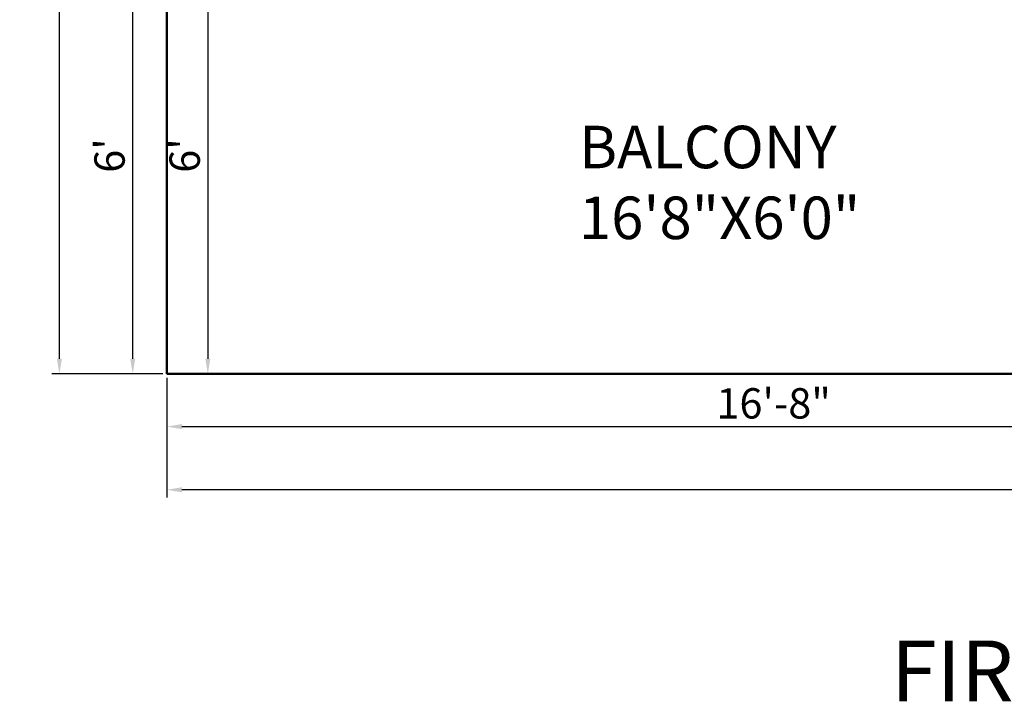
# Model space of a CAD drawing. Units: inches. Extents: x 3064 to 19385, y 846 to 15425.
# Tile 92 of 108: x 7502 to 7664, y 850 to 963. Entities that reach past the tile are written whole.
import ezdxf

# ---------------------------------------------------------------- set-up
doc = ezdxf.new("R2010")
doc.units = ezdxf.units.IN
for name, color, linetype, lineweight in [('A-ANNO-DIMS', 2, 'Continuous', 18), ('A-ANNO-TEXT', 7, 'Continuous', 25), ('A-AREA-IDEN', 3, 'Continuous', 18), ('A-WALL', 7, 'Continuous', 50)]:
    doc.layers.add(name, color=color, linetype=linetype, lineweight=lineweight)
doc.styles.get("Standard").update_dxf_attribs({"font": 'arial.ttf'})
doc.dimstyles.new('ISO-25', dxfattribs={"dimtxt": 9, "dimasz": 2.5, "dimexe": 1.25, "dimexo": 0.625, "dimtad": 1, "dimdec": 1, "dimlunit": 3, "dimtxsty": 'Standard', "dimcen": 2.5, "dimadec": 0, "dimazin": 0, "dimtfac": 1, "dimtdec": 1, "dimtmove": 0, "dimatfit": 3, "dimfxl": 1, "dimarcsym": 0})

# ---------------------------------------------------------------- blocks, each defined once
blk = doc.blocks.new('*D316')
at = {"layer": 'A-ANNO-DIMS', "color": 0, "lineweight": -2, "transparency": 16777216}
for p, q in [((7525.62, 976.34), (7519.4, 976.34)), ((7520.65, 906.84), (7520.65, 973.84)), ((7525.62, 904.34), (7519.4, 904.34))]:
    blk.add_line(p, q, dxfattribs=at)
at = {"layer": 'A-ANNO-DIMS', "color": 0, "transparency": 16777216}
for points in [[(7520.23, 973.84), (7521.06, 973.84), (7520.65, 976.34)], [(7520.23, 906.84), (7521.06, 906.84), (7520.65, 904.34)]]:
    blk.add_solid(points, dxfattribs=at)
at = {"layer": 'Defpoints', "color": 0, "transparency": 16777216}
for p in [(7520.65, 976.34), (7526.25, 976.34), (7526.25, 904.34)]:
    blk.add_point(p, dxfattribs=at)
at = {"layer": 'A-ANNO-DIMS', "color": 0, "transparency": 16777216, "insert": (7517.47, 940.34), "char_height": 5, "attachment_point": 5, "rotation": 90}
blk.add_mtext("6'", dxfattribs=at)
blk = doc.blocks.new('*D324')
at = {"layer": 'A-ANNO-DIMS', "color": 0, "lineweight": -2, "transparency": 16777216}
for p, q in [((7525.62, 1396.34), (7507.31, 1396.34)), ((7508.56, 906.84), (7508.56, 1393.84)), ((7525.62, 904.34), (7507.31, 904.34))]:
    blk.add_line(p, q, dxfattribs=at)
at = {"layer": 'A-ANNO-DIMS', "color": 0, "transparency": 16777216}
for points in [[(7508.15, 1393.84), (7508.98, 1393.84), (7508.56, 1396.34)], [(7508.15, 906.84), (7508.98, 906.84), (7508.56, 904.34)]]:
    blk.add_solid(points, dxfattribs=at)
at = {"layer": 'Defpoints', "color": 0, "transparency": 16777216}
for p in [(7508.56, 1396.34), (7526.25, 1396.34), (7526.25, 904.34)]:
    blk.add_point(p, dxfattribs=at)
at = {"layer": 'A-ANNO-DIMS', "color": 0, "transparency": 16777216, "insert": (7505.43, 1150.34), "char_height": 5, "attachment_point": 5, "rotation": 90}
blk.add_mtext("41'", dxfattribs=at)
blk = doc.blocks.new('*D325')
at = {"layer": 'A-ANNO-DIMS', "color": 0, "lineweight": -2, "transparency": 16777216}
for p, q in [((7526.25, 903.71), (7526.25, 894.42)), ((7726.25, 903.71), (7726.25, 894.42)), ((7528.75, 895.67), (7723.75, 895.67))]:
    blk.add_line(p, q, dxfattribs=at)
at = {"layer": 'A-ANNO-DIMS', "color": 0, "transparency": 16777216}
for points in [[(7528.75, 896.08), (7528.75, 895.25), (7526.25, 895.67)], [(7723.75, 896.08), (7723.75, 895.25), (7726.25, 895.67)]]:
    blk.add_solid(points, dxfattribs=at)
at = {"layer": 'Defpoints', "color": 0, "transparency": 16777216}
for p in [(7526.25, 904.34), (7726.25, 904.34), (7726.25, 895.67)]:
    blk.add_point(p, dxfattribs=at)
at = {"layer": 'A-ANNO-DIMS', "color": 0, "transparency": 16777216, "insert": (7626.25, 898.85), "char_height": 5, "attachment_point": 5}
blk.add_mtext('16\'-8"', dxfattribs=at)
blk = doc.blocks.new('*D224')
at = {"layer": 'A-ANNO-DIMS', "color": 0, "lineweight": -2, "transparency": 16777216}
for p, q in [((7526.25, 903.71), (7526.25, 884.01)), ((7868.25, 903.71), (7868.25, 884.01)), ((7865.75, 885.26), (7528.75, 885.26))]:
    blk.add_line(p, q, dxfattribs=at)
at = {"layer": 'A-ANNO-DIMS', "color": 0, "transparency": 16777216}
for points in [[(7528.75, 885.67), (7528.75, 884.84), (7526.25, 885.26)], [(7865.75, 885.67), (7865.75, 884.84), (7868.25, 885.26)]]:
    blk.add_solid(points, dxfattribs=at)
at = {"layer": 'Defpoints', "color": 0, "transparency": 16777216}
for p in [(7526.25, 904.34), (7868.25, 904.34), (7526.25, 885.26)]:
    blk.add_point(p, dxfattribs=at)
at = {"layer": 'A-ANNO-DIMS', "color": 0, "transparency": 16777216, "insert": (7697.25, 888.43), "char_height": 5, "attachment_point": 5}
blk.add_mtext('28\'-6"', dxfattribs=at)
blk = doc.blocks.new('*D220')
at = {"layer": 'A-ANNO-DIMS', "color": 0, "lineweight": -2, "transparency": 16777216}
for p, q in [((7526.87, 976.34), (7534.27, 976.34)), ((7533.02, 973.84), (7533.02, 906.84)), ((7526.87, 904.34), (7534.27, 904.34))]:
    blk.add_line(p, q, dxfattribs=at)
at = {"layer": 'A-ANNO-DIMS', "color": 0, "transparency": 16777216}
for points in [[(7532.61, 973.84), (7533.44, 973.84), (7533.02, 976.34)], [(7532.61, 906.84), (7533.44, 906.84), (7533.02, 904.34)]]:
    blk.add_solid(points, dxfattribs=at)
at = {"layer": 'Defpoints', "color": 0, "transparency": 16777216}
for p in [(7526.25, 976.34), (7526.25, 904.34), (7533.02, 904.34)]:
    blk.add_point(p, dxfattribs=at)
at = {"layer": 'A-ANNO-DIMS', "color": 0, "transparency": 16777216, "insert": (7529.85, 940.34), "char_height": 5, "attachment_point": 5, "rotation": 90}
blk.add_mtext("6'", dxfattribs=at)

msp = doc.modelspace()

# ---------------------------------------------------------------- linework, layer by layer
at = {"layer": 'A-WALL'}
for p, q in [((7526.25, 976.34), (7526.25, 904.34)), ((7526.25, 904.34), (7868.25, 904.34))]:
    msp.add_line(p, q, dxfattribs=at)

# ---------------------------------------------------------------- texts
at = {"layer": 'A-ANNO-TEXT', "insert": (7645.59, 860.41), "char_height": 10, "attachment_point": 1}
msp.add_mtext_dynamic_manual_height_columns('FIRST FLOOR PLAN', width=200.9739, gutter_width=12.5, heights=[0], dxfattribs=at)
at = {"layer": 'A-AREA-IDEN', "insert": (7594.18, 945.24), "char_height": 7, "attachment_point": 1}
msp.add_mtext_dynamic_manual_height_columns('BALCONY\\P16\'8"X6\'0"', width=67.5924, gutter_width=12.5, heights=[0], dxfattribs=at)

# ---------------------------------------------------------------- dimensions: what is measured, and where the dimension line sits
at = {"layer": 'A-ANNO-DIMS'}
for base, p1, p2, picture, middle in [((7508.56, 1396.34), (7526.25, 904.34), (7526.25, 1396.34), '*D324', (7505.43, 1150.34)), ((7520.65, 976.34), (7526.25, 904.34), (7526.25, 976.34), '*D316', (7517.47, 940.34)), ((7533.02, 904.34), (7526.25, 976.34), (7526.25, 904.34), '*D220', (7529.85, 940.34))]:
    dim = msp.add_linear_dim(base=base, p1=p1, p2=p2, angle=90, dimstyle='ISO-25', override={"dimtxt": 5, "dimclrd": 0, "dimclre": 0, "dimclrt": 0}, dxfattribs=at)
    dim.commit()
    dim.dimension.update_dxf_attribs({"geometry": picture, "text_midpoint": middle})
for base, p1, p2, picture, middle in [((7726.25, 895.67), (7526.25, 904.34), (7726.25, 904.34), '*D325', (7626.25, 898.85)), ((7526.25, 885.26), (7868.25, 904.34), (7526.25, 904.34), '*D224', (7697.25, 888.43))]:
    dim = msp.add_linear_dim(base=base, p1=p1, p2=p2, dimstyle='ISO-25', override={"dimtxt": 5, "dimclrd": 0, "dimclre": 0, "dimclrt": 0}, dxfattribs=at)
    dim.commit()
    dim.dimension.update_dxf_attribs({"geometry": picture, "text_midpoint": middle})

doc.saveas('drawing.dxf')
